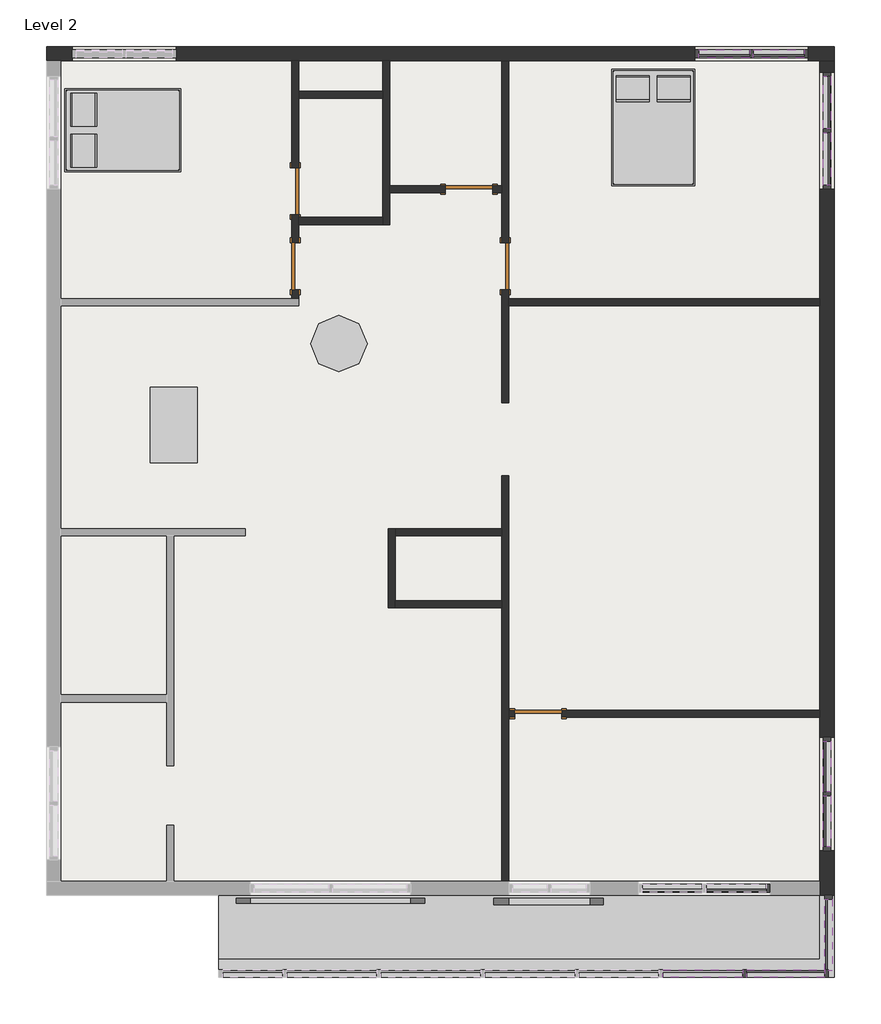
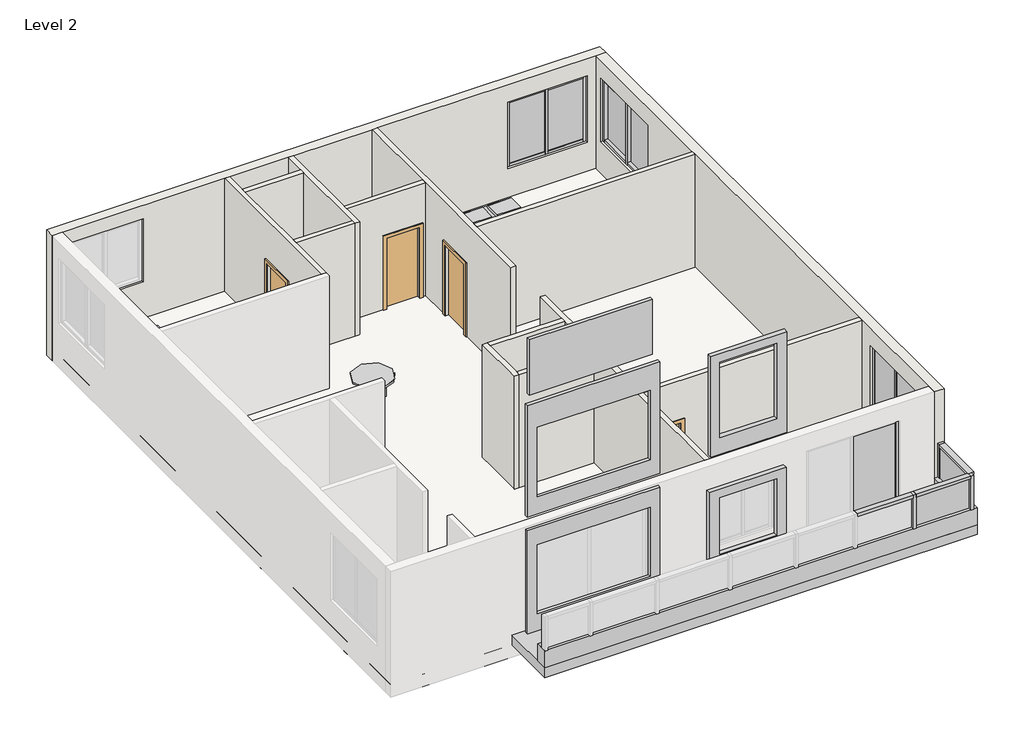
# One storey, part 2 of 2: 30 members, 14 walls, 9 plates, 5 doors, 4 furniture elements, 3 proxies, 1 roof.
"""IFC4 building model written with IfcOpenShell, lengths in millimetres."""

from ifc_helpers import new_model, si_unit, frame, origin, place, context, project, spatial, polyline, outline, extrude, faceted_brep, transform, mapped, element, save
from components import generic_models_10_generic_models_10_e6df43e6, generic_models_11_generic_models_11_8cdfda78, generic_models_4_generic_models_4_9f1effd6, door_f2b275c1, door_d8f5dbb5, furniture_b58f7881, furniture_acc2807d, furniture_52f35bf4, member_c17f1be2, member_7ceeb836, member_9efbbc5c, member_8b2b7717, member_31190633, member_ed313243, member_872f6578, member_8cf20c82, member_801a2072, member_dae9f1c3, member_bf3bc0fd, member_a6f19fa4, member_8ac64e86, member_d7462ea5, member_4edd9ee4, member_1e0ac351, system_panel_glazed_171f6735, system_panel_glazed_e9dc8a15, system_panel_glazed_abee1f72, system_panel_glazed_a27b9eb0, system_panel_glazed_117fd4c3, system_panel_glazed_6fb9d5dc

model = new_model("IFC4")

# Units and contexts
model_context = context("Model", 3, world=origin())
ifc_project = project(units=[si_unit("LENGTHUNIT", "METRE", prefix="MILLI")], contexts=[model_context])

# Site, building, storey
site = spatial("IfcSite", under=ifc_project)
building = spatial("IfcBuilding", under=site)
storey = spatial("IfcBuildingStorey", under=building, Name="Level 2", Elevation=3048.0)

# Proxies
placement = place(None, origin())
generic_models_10_generic_models_10_shape = generic_models_10_generic_models_10_e6df43e6(model_context)
element("IfcBuildingElementProxy", 1, Name="Generic Models 10 : Generic Models 10", ObjectType="Generic Models 10 : Generic Models 10", at=placement, inside=storey, context=model_context, shape_type="MappedRepresentation", body=[
    mapped(generic_models_10_generic_models_10_shape, transform((0.0, 0.0, 0.0), x_axis=(1.0, 0.0, 0.0), y_axis=(0.0, 1.0, 0.0), z_axis=(0.0, 0.0, 1.0))),
])
generic_models_11_generic_models_11_shape = generic_models_11_generic_models_11_8cdfda78(model_context)
element("IfcBuildingElementProxy", 2, Name="Generic Models 11 : Generic Models 11", ObjectType="Generic Models 11 : Generic Models 11", at=placement, inside=storey, context=model_context, shape_type="MappedRepresentation", body=[
    mapped(generic_models_11_generic_models_11_shape, transform((0.0, 0.0, 0.0), x_axis=(1.0, 0.0, 0.0), y_axis=(0.0, 1.0, 0.0), z_axis=(0.0, 0.0, 1.0))),
])
generic_models_4_generic_models_4_shape = generic_models_4_generic_models_4_9f1effd6(model_context)
element("IfcBuildingElementProxy", 3, Name="Generic Models 4 : Generic Models 4", ObjectType="Generic Models 4 : Generic Models 4", at=placement, inside=storey, context=model_context, shape_type="MappedRepresentation", body=[
    mapped(generic_models_4_generic_models_4_shape, transform((0.0, 0.0, 0.0), x_axis=(1.0, 0.0, 0.0), y_axis=(0.0, 1.0, 0.0), z_axis=(0.0, 0.0, 1.0))),
])

# Doors
door_shape = door_f2b275c1(model_context)
element("IfcDoor", 4, ObjectType="Single-Flush : 30\" x 80\"", at=placement, inside=storey, context=model_context, shape_type="MappedRepresentation", body=[
    mapped(door_shape, transform((-14978.0695233, -3968.4252569, 3048.0), x_axis=(0.0, -1.0, 0.0), y_axis=(1.0, 0.0, 0.0), z_axis=(0.0, 0.0, 1.0))),
])
element("IfcDoor", 5, ObjectType="Single-Flush : 30\" x 80\"", at=placement, inside=storey, context=model_context, shape_type="MappedRepresentation", body=[
    mapped(door_shape, transform((-11053.7695233, -11201.0752569, 3048.0), x_axis=(-1.0, 0.0, 0.0), y_axis=(0.0, -1.0, 0.0), z_axis=(0.0, 0.0, 1.0))),
])
door_2_shape = door_d8f5dbb5(model_context)
element("IfcDoor", 6, ObjectType="Single-Flush : 30\" x 80\"", at=placement, inside=storey, context=model_context, shape_type="MappedRepresentation", body=[
    mapped(door_2_shape, transform((-14978.0695233, -2755.5752569, 3048.0), x_axis=(0.0, -1.0, 0.0), y_axis=(1.0, 0.0, 0.0), z_axis=(0.0, 0.0, 1.0))),
])
element("IfcDoor", 7, ObjectType="Single-Flush : 30\" x 80\"", at=placement, inside=storey, context=model_context, shape_type="MappedRepresentation", body=[
    mapped(door_2_shape, transform((-12171.3695233, -2723.8252569, 3048.0), x_axis=(1.0, 0.0, 0.0), y_axis=(0.0, 1.0, 0.0), z_axis=(0.0, 0.0, 1.0))),
])
element("IfcDoor", 8, ObjectType="Single-Flush : 30\" x 80\"", at=placement, inside=storey, context=model_context, shape_type="MappedRepresentation", body=[
    mapped(door_2_shape, transform((-11587.1695233, -3968.4252569, 3048.0), x_axis=(0.0, -1.0, 0.0), y_axis=(1.0, 0.0, 0.0), z_axis=(0.0, 0.0, 1.0))),
])

# Furniture
furniture_shape = furniture_b58f7881(model_context)
element("IfcFurniture", 9, ObjectType="Bed-Box : Double 53\" x 74\"", at=placement, inside=storey, context=model_context, shape_type="MappedRepresentation", body=[
    mapped(furniture_shape, transform((-18000.1490315, -2110.4777159, 3048.0), x_axis=(0.0, 1.0, 0.0), y_axis=(-1.0, 0.0, 0.0), z_axis=(0.0, 0.0, 1.0))),
])
element("IfcFurniture", 10, ObjectType="Bed-Box : Double 53\" x 74\"", at=placement, inside=storey, context=model_context, shape_type="MappedRepresentation", body=[
    mapped(furniture_shape, transform((-9532.3719823, -1492.4457487, 3048.0), x_axis=(1.0, 0.0, 0.0), y_axis=(0.0, 1.0, 0.0), z_axis=(0.0, 0.0, 1.0))),
])
furniture_2_shape = furniture_acc2807d(model_context)
element("IfcFurniture", 11, ObjectType="Table-Coffee Rectangular : 48\" x 30\"", at=placement, inside=storey, context=model_context, shape_type="MappedRepresentation", body=[
    mapped(furniture_2_shape, transform((-16570.6086915, -7147.1588872, 3048.0), x_axis=(0.0, 1.0, 0.0), y_axis=(-1.0, 0.0, 0.0), z_axis=(0.0, 0.0, 1.0))),
])
furniture_3_shape = furniture_52f35bf4(model_context)
element("IfcFurniture", 12, ObjectType="Table-Dining Round w Chairs : 36\" Diameter", at=placement, inside=storey, context=model_context, shape_type="MappedRepresentation", body=[
    mapped(furniture_3_shape, transform((-14376.9014905, -5034.4965684, 3048.0), x_axis=(1.0, 0.0, 0.0), y_axis=(0.0, 1.0, 0.0), z_axis=(0.0, 0.0, 1.0))),
])

# Members
member_shape = member_c17f1be2(model_context)
element("IfcMember", 13, ObjectType="Rectangular Mullion : 2.5\" x 5\" rectangular", at=placement, inside=storey, context=model_context, shape_type="MappedRepresentation", body=[
    mapped(member_shape, transform((-6386.5195233, -12528.2252569, 5666.1206618), x_axis=(0.0, 0.0, 1.0), y_axis=(1.0, 0.0, 0.0), z_axis=(0.0, 1.0, 0.0))),
])
element("IfcMember", 14, ObjectType="Rectangular Mullion : 2.5\" x 5\" rectangular", at=placement, inside=storey, context=model_context, shape_type="MappedRepresentation", body=[
    mapped(member_shape, transform((-6386.5195233, -11645.5752569, 5666.1206618), x_axis=(0.0, 0.0, 1.0), y_axis=(1.0, 0.0, 0.0), z_axis=(0.0, 1.0, 0.0))),
])
element("IfcMember", 15, ObjectType="Rectangular Mullion : 2.5\" x 5\" rectangular", at=placement, inside=storey, context=model_context, shape_type="MappedRepresentation", body=[
    mapped(member_shape, transform((-7573.9695233, -533.0752569, 5665.5630384), x_axis=(0.0, 0.0, 1.0), y_axis=(0.0, 1.0, 0.0), z_axis=(-1.0, 0.0, 0.0))),
])
element("IfcMember", 16, ObjectType="Rectangular Mullion : 2.5\" x 5\" rectangular", at=placement, inside=storey, context=model_context, shape_type="MappedRepresentation", body=[
    mapped(member_shape, transform((-8456.6195233, -533.0752569, 5665.5630384), x_axis=(0.0, 0.0, 1.0), y_axis=(0.0, 1.0, 0.0), z_axis=(-1.0, 0.0, 0.0))),
])
element("IfcMember", 17, ObjectType="Rectangular Mullion : 2.5\" x 5\" rectangular", at=placement, inside=storey, context=model_context, shape_type="MappedRepresentation", body=[
    mapped(member_shape, transform((-6386.5195233, -12464.7252569, 4092.4481408), x_axis=(0.0, 0.0, -1.0), y_axis=(1.0, 0.0, 0.0), z_axis=(0.0, -1.0, 0.0))),
])
element("IfcMember", 18, ObjectType="Rectangular Mullion : 2.5\" x 5\" rectangular", at=placement, inside=storey, context=model_context, shape_type="MappedRepresentation", body=[
    mapped(member_shape, transform((-6386.5195233, -13347.3752569, 4092.4481408), x_axis=(0.0, 0.0, -1.0), y_axis=(1.0, 0.0, 0.0), z_axis=(0.0, -1.0, 0.0))),
])
element("IfcMember", 19, ObjectType="Rectangular Mullion : 2.5\" x 5\" rectangular", at=placement, inside=storey, context=model_context, shape_type="MappedRepresentation", body=[
    mapped(member_shape, transform((-7637.4695233, -533.0752569, 4055.4970292), x_axis=(0.0, 0.0, -1.0), y_axis=(0.0, 1.0, 0.0), z_axis=(1.0, 0.0, 0.0))),
])
element("IfcMember", 20, ObjectType="Rectangular Mullion : 2.5\" x 5\" rectangular", at=placement, inside=storey, context=model_context, shape_type="MappedRepresentation", body=[
    mapped(member_shape, transform((-6754.8195233, -533.0752569, 4055.4970292), x_axis=(0.0, 0.0, -1.0), y_axis=(0.0, 1.0, 0.0), z_axis=(1.0, 0.0, 0.0))),
])
member_2_shape = member_7ceeb836(model_context)
element("IfcMember", 21, ObjectType="Rectangular Mullion : 2.5\" x 5\" rectangular", at=placement, inside=storey, context=model_context, shape_type="MappedRepresentation", body=[
    mapped(member_2_shape, transform((-6386.5195233, -12496.4752569, 4092.4481408), x_axis=(0.0, 1.0, 0.0), y_axis=(1.0, 0.0, 0.0), z_axis=(0.0, 0.0, -1.0))),
])
member_3_shape = member_9efbbc5c(model_context)
element("IfcMember", 22, ObjectType="Rectangular Mullion : 2.5\" x 5\" rectangular", at=placement, inside=storey, context=model_context, shape_type="MappedRepresentation", body=[
    mapped(member_3_shape, transform((-6386.5195233, -11582.0752569, 4092.4481408), x_axis=(0.0, 1.0, 0.0), y_axis=(1.0, 0.0, 0.0), z_axis=(0.0, 0.0, -1.0))),
])
element("IfcMember", 23, ObjectType="Rectangular Mullion : 2.5\" x 5\" rectangular", at=placement, inside=storey, context=model_context, shape_type="MappedRepresentation", body=[
    mapped(member_3_shape, transform((-6386.5195233, -13410.8752569, 5666.1206618), x_axis=(0.0, -1.0, 0.0), y_axis=(1.0, 0.0, 0.0), z_axis=(0.0, 0.0, 1.0))),
])
member_4_shape = member_8b2b7717(model_context)
element("IfcMember", 24, ObjectType="Rectangular Mullion : 2.5\" x 5\" rectangular", at=placement, inside=storey, context=model_context, shape_type="MappedRepresentation", body=[
    mapped(member_4_shape, transform((-6386.5195233, -1749.1002569, 5662.3065021), x_axis=(0.0, 0.0, 1.0), y_axis=(-1.0, 0.0, 0.0), z_axis=(0.0, -1.0, 0.0))),
])
element("IfcMember", 25, ObjectType="Rectangular Mullion : 2.5\" x 5\" rectangular", at=placement, inside=storey, context=model_context, shape_type="MappedRepresentation", body=[
    mapped(member_4_shape, transform((-6386.5195233, -2660.3252569, 5662.3065021), x_axis=(0.0, 0.0, 1.0), y_axis=(-1.0, 0.0, 0.0), z_axis=(0.0, -1.0, 0.0))),
])
member_5_shape = member_31190633(model_context)
element("IfcMember", 26, ObjectType="Rectangular Mullion : 2.5\" x 5\" rectangular", at=placement, inside=storey, context=model_context, shape_type="MappedRepresentation", body=[
    mapped(member_5_shape, transform((-6386.5195233, -1780.8502569, 4118.2676492), x_axis=(0.0, -1.0, 0.0), y_axis=(-1.0, 0.0, 0.0), z_axis=(0.0, 0.0, -1.0))),
])
element("IfcMember", 27, ObjectType="Rectangular Mullion : 2.5\" x 5\" rectangular", at=placement, inside=storey, context=model_context, shape_type="MappedRepresentation", body=[
    mapped(member_4_shape, transform((-6386.5195233, -1812.6002569, 4118.2676492), x_axis=(0.0, 0.0, -1.0), y_axis=(-1.0, 0.0, 0.0), z_axis=(0.0, 1.0, 0.0))),
])
element("IfcMember", 28, ObjectType="Rectangular Mullion : 2.5\" x 5\" rectangular", at=placement, inside=storey, context=model_context, shape_type="MappedRepresentation", body=[
    mapped(member_4_shape, transform((-6386.5195233, -901.3752569, 4118.2676492), x_axis=(0.0, 0.0, -1.0), y_axis=(-1.0, 0.0, 0.0), z_axis=(0.0, 1.0, 0.0))),
])
member_6_shape = member_ed313243(model_context)
element("IfcMember", 29, ObjectType="Rectangular Mullion : 2.5\" x 5\" rectangular", at=placement, inside=storey, context=model_context, shape_type="MappedRepresentation", body=[
    mapped(member_6_shape, transform((-6386.5195233, -837.8752569, 5662.3065021), x_axis=(0.0, 1.0, 0.0), y_axis=(-1.0, 0.0, 0.0), z_axis=(0.0, 0.0, 1.0))),
])
element("IfcMember", 30, ObjectType="Rectangular Mullion : 2.5\" x 5\" rectangular", at=placement, inside=storey, context=model_context, shape_type="MappedRepresentation", body=[
    mapped(member_6_shape, transform((-6386.5195233, -2723.8252569, 4118.2676492), x_axis=(0.0, -1.0, 0.0), y_axis=(-1.0, 0.0, 0.0), z_axis=(0.0, 0.0, -1.0))),
])
member_7_shape = member_872f6578(model_context)
element("IfcMember", 31, ObjectType="Rectangular Mullion : 2.5\" x 5\" rectangular", at=placement, inside=storey, context=model_context, shape_type="MappedRepresentation", body=[
    mapped(member_7_shape, transform((-7605.7195233, -533.0752569, 4055.4970292), x_axis=(-1.0, 0.0, 0.0), y_axis=(0.0, 1.0, 0.0), z_axis=(0.0, 0.0, -1.0))),
])
member_8_shape = member_8cf20c82(model_context)
element("IfcMember", 32, ObjectType="Rectangular Mullion : 2.5\" x 5\" rectangular", at=placement, inside=storey, context=model_context, shape_type="MappedRepresentation", body=[
    mapped(member_8_shape, transform((-8520.1195233, -533.0752569, 4055.4970292), x_axis=(-1.0, 0.0, 0.0), y_axis=(0.0, 1.0, 0.0), z_axis=(0.0, 0.0, -1.0))),
])
element("IfcMember", 33, ObjectType="Rectangular Mullion : 2.5\" x 5\" rectangular", at=placement, inside=storey, context=model_context, shape_type="MappedRepresentation", body=[
    mapped(member_8_shape, transform((-6691.3195233, -533.0752569, 5665.5630384), x_axis=(1.0, 0.0, 0.0), y_axis=(0.0, 1.0, 0.0), z_axis=(0.0, 0.0, 1.0))),
])
member_9_shape = member_801a2072(model_context)
element("IfcMember", 34, ObjectType="Rectangular Mullion : 2.5\" x 5\" rectangular", at=placement, inside=storey, context=model_context, shape_type="MappedRepresentation", body=[
    mapped(member_9_shape, transform((-8399.4695233, -14020.4752569, 3693.4399111), x_axis=(0.0, 0.0, -1.0), y_axis=(0.0, 1.0, 0.0), z_axis=(1.0, 0.0, 0.0))),
])
element("IfcMember", 35, ObjectType="Rectangular Mullion : 2.5\" x 5\" rectangular", at=placement, inside=storey, context=model_context, shape_type="MappedRepresentation", body=[
    mapped(member_9_shape, transform((-7364.4195233, -14020.4752569, 3693.4399111), x_axis=(0.0, 0.0, -1.0), y_axis=(0.0, 1.0, 0.0), z_axis=(1.0, 0.0, 0.0))),
])
member_10_shape = member_dae9f1c3(model_context)
element("IfcMember", 36, ObjectType="Rectangular Mullion : 2.5\" x 5\" rectangular", at=placement, inside=storey, context=model_context, shape_type="MappedRepresentation", body=[
    mapped(member_10_shape, transform((-7300.9195233, -14020.4752569, 5682.139627), x_axis=(1.0, 0.0, 0.0), y_axis=(0.0, 1.0, 0.0), z_axis=(0.0, 0.0, 1.0))),
])
member_11_shape = member_bf3bc0fd(model_context)
element("IfcMember", 37, ObjectType="Rectangular Mullion : 2.5\" x 5\" rectangular", at=placement, inside=storey, context=model_context, shape_type="MappedRepresentation", body=[
    mapped(member_11_shape, transform((-7748.4379121, -15398.1130528, 4822.8286641), x_axis=(0.0, 0.0, 1.0), y_axis=(0.0, -1.0, 0.0), z_axis=(1.0, 0.0, 0.0))),
])
member_12_shape = member_a6f19fa4(model_context)
element("IfcMember", 38, ObjectType="Rectangular Mullion : 2.5\" x 5\" rectangular", at=placement, inside=storey, context=model_context, shape_type="MappedRepresentation", body=[
    mapped(member_12_shape, transform((-6425.5212454, -15398.1130528, 4822.8286641), x_axis=(0.0, 0.0, 1.0), y_axis=(0.0, -1.0, 0.0), z_axis=(1.0, 0.0, 0.0))),
])
member_13_shape = member_8ac64e86(model_context)
element("IfcMember", 39, ObjectType="Rectangular Mullion : 2.5\" x 5\" rectangular", at=placement, inside=storey, context=model_context, shape_type="MappedRepresentation", body=[
    mapped(member_13_shape, transform((-6362.0212454, -15398.1130528, 4001.8016497), x_axis=(1.0, 0.0, 0.0), y_axis=(0.0, -1.0, 0.0), z_axis=(0.0, 0.0, -1.0))),
])
member_14_shape = member_d7462ea5(model_context)
element("IfcMember", 40, ObjectType="Rectangular Mullion : 2.5\" x 5\" rectangular", at=placement, inside=storey, context=model_context, shape_type="MappedRepresentation", body=[
    mapped(member_14_shape, transform((-7716.6879121, -15398.1130528, 4001.8016497), x_axis=(1.0, 0.0, 0.0), y_axis=(0.0, -1.0, 0.0), z_axis=(0.0, 0.0, -1.0))),
])
member_15_shape = member_4edd9ee4(model_context)
element("IfcMember", 41, ObjectType="Rectangular Mullion : 2.5\" x 5\" rectangular", at=placement, inside=storey, context=model_context, shape_type="MappedRepresentation", body=[
    mapped(member_15_shape, transform((-6362.0212454, -14134.7752569, 4001.8016497), x_axis=(0.0, 1.0, 0.0), y_axis=(1.0, 0.0, 0.0), z_axis=(0.0, 0.0, -1.0))),
])
member_16_shape = member_1e0ac351(model_context)
element("IfcMember", 42, ObjectType="Rectangular Mullion : 2.5\" x 5\" rectangular", at=placement, inside=storey, context=model_context, shape_type="MappedRepresentation", body=[
    mapped(member_16_shape, transform((-6362.0212454, -14198.2752569, 4825.345459), x_axis=(0.0, 0.0, 1.0), y_axis=(1.0, 0.0, 0.0), z_axis=(0.0, 1.0, 0.0))),
])

# Plates
system_panel_glazed_shape = system_panel_glazed_171f6735(model_context)
element("IfcPlate", 43, ObjectType="System Panel : Glazed", at=placement, inside=storey, context=model_context, shape_type="MappedRepresentation", body=[
    mapped(system_panel_glazed_shape, transform((-6386.5195233, -12937.8002569, 4155.9481408), x_axis=(0.0, 1.0, 0.0), y_axis=(-1.0, 0.0, 0.0), z_axis=(0.0, 0.0, 1.0))),
])
element("IfcPlate", 44, ObjectType="System Panel : Glazed", at=placement, inside=storey, context=model_context, shape_type="MappedRepresentation", body=[
    mapped(system_panel_glazed_shape, transform((-6386.5195233, -12055.1502569, 4155.9481408), x_axis=(0.0, 1.0, 0.0), y_axis=(-1.0, 0.0, 0.0), z_axis=(0.0, 0.0, 1.0))),
])
system_panel_glazed_2_shape = system_panel_glazed_e9dc8a15(model_context)
element("IfcPlate", 45, ObjectType="System Panel : Glazed", at=placement, inside=storey, context=model_context, shape_type="MappedRepresentation", body=[
    mapped(system_panel_glazed_2_shape, transform((-6386.5195233, -1325.2377569, 4181.7676492), x_axis=(0.0, -1.0, 0.0), y_axis=(1.0, 0.0, 0.0), z_axis=(0.0, 0.0, 1.0))),
])
element("IfcPlate", 46, ObjectType="System Panel : Glazed", at=placement, inside=storey, context=model_context, shape_type="MappedRepresentation", body=[
    mapped(system_panel_glazed_2_shape, transform((-6386.5195233, -2236.4627569, 4181.7676492), x_axis=(0.0, -1.0, 0.0), y_axis=(1.0, 0.0, 0.0), z_axis=(0.0, 0.0, 1.0))),
])
system_panel_glazed_3_shape = system_panel_glazed_abee1f72(model_context)
element("IfcPlate", 47, ObjectType="System Panel : Glazed", at=placement, inside=storey, context=model_context, shape_type="MappedRepresentation", body=[
    mapped(system_panel_glazed_3_shape, transform((-7164.3945233, -533.0752569, 4118.9970292), x_axis=(-1.0, 0.0, 0.0), y_axis=(0.0, -1.0, 0.0), z_axis=(0.0, 0.0, 1.0))),
])
element("IfcPlate", 48, ObjectType="System Panel : Glazed", at=placement, inside=storey, context=model_context, shape_type="MappedRepresentation", body=[
    mapped(system_panel_glazed_3_shape, transform((-8047.0445233, -533.0752569, 4118.9970292), x_axis=(-1.0, 0.0, 0.0), y_axis=(0.0, -1.0, 0.0), z_axis=(0.0, 0.0, 1.0))),
])
system_panel_glazed_4_shape = system_panel_glazed_a27b9eb0(model_context)
element("IfcPlate", 49, ObjectType="System Panel : Glazed", at=placement, inside=storey, context=model_context, shape_type="MappedRepresentation", body=[
    mapped(system_panel_glazed_4_shape, transform((-7850.1945233, -14020.4752569, 3756.9399111), x_axis=(-1.0, 0.0, 0.0), y_axis=(0.0, -1.0, 0.0), z_axis=(0.0, 0.0, 1.0))),
])
system_panel_glazed_5_shape = system_panel_glazed_117fd4c3(model_context)
element("IfcPlate", 50, ObjectType="System Panel : Glazed", at=placement, inside=storey, context=model_context, shape_type="MappedRepresentation", body=[
    mapped(system_panel_glazed_5_shape, transform((-7055.2295788, -15398.1130528, 4001.8016497), x_axis=(1.0, 0.0, 0.0), y_axis=(0.0, 1.0, 0.0), z_axis=(0.0, 0.0, 1.0))),
])
system_panel_glazed_6_shape = system_panel_glazed_6fb9d5dc(model_context)
element("IfcPlate", 51, ObjectType="System Panel : Glazed", at=placement, inside=storey, context=model_context, shape_type="MappedRepresentation", body=[
    mapped(system_panel_glazed_6_shape, transform((-6362.0212454, -14775.9691549, 4001.8016497), x_axis=(0.0, 1.0, 0.0), y_axis=(-1.0, 0.0, 0.0), z_axis=(0.0, 0.0, 1.0))),
])

# Roof
element("IfcRoof", 52, ObjectType="Generic - 12\"", at=placement, inside=storey, context=model_context, shape_type="SweptSolid", body=[
    extrude(outline(polyline([(-18997.6195233, -418.7752569), (-6272.2195233, -418.7752569), (-6272.2195233, -14134.7752569), (-18997.6195233, -14134.7752569), (-18997.6195233, -418.7752569)])), frame((0.0, 0.0, 3048.0), z_axis=(0.0, 0.0, 1.0), x_axis=(1.0, 0.0, 0.0)), (0.0, 0.0, 1.0), 304.8),
])

# Walls
element("IfcWall", 53, ObjectType="4.5\"", at=placement, inside=storey, context=model_context, shape_type="Brep", body=[
    faceted_brep([(-11530.0195233, -13906.1752569, 3048.0), (-11530.0195233, -11258.2252569, 3048.0), (-11530.0195233, -11143.9252569, 3048.0), (-11530.0195233, -7352.9752569, 3048.0), (-11530.0195233, -7352.9752569, 6096.0), (-11530.0195233, -11143.9252569, 6096.0), (-11530.0195233, -11258.2252569, 6096.0), (-11530.0195233, -13906.1752569, 6096.0), (-11644.3195233, -13906.1752569, 3048.0), (-11644.3195233, -13906.1752569, 6096.0), (-11644.3195233, -9486.5752569, 6096.0), (-11644.3195233, -9372.2752569, 6096.0), (-11644.3195233, -8324.5252569, 6096.0), (-11644.3195233, -8210.2252569, 6096.0), (-11644.3195233, -7352.9752569, 6096.0), (-11644.3195233, -7352.9752569, 3048.0), (-11644.3195233, -8210.2252569, 3048.0), (-11644.3195233, -8324.5252569, 3048.0), (-11644.3195233, -9372.2752569, 3048.0), (-11644.3195233, -9486.5752569, 3048.0)], [[[0, 1, 2, 3, 4, 5, 6, 7]], [[8, 9, 10, 11, 12, 13, 14, 15, 16, 17, 18, 19]], [[3, 2, 1, 0, 8, 19, 18, 17, 16, 15]], [[4, 3, 15, 14]], [[7, 6, 5, 4, 14, 13, 12, 11, 10, 9]], [[0, 7, 9, 8]]]),
])
element("IfcWall", 54, ObjectType="4.5\"", at=placement, inside=storey, context=model_context, shape_type="SweptSolid", body=[
    extrude(outline(polyline([(3048.0, -11530.0195233), (3048.0, -11434.7695233), (5080.0, -11434.7695233), (5080.0, -10672.7695233), (3048.0, -10672.7695233), (3048.0, -6500.8195233), (6096.0, -6500.8195233), (6096.0, -11530.0195233), (3048.0, -11530.0195233)])), frame((0.0, -11258.2252569, 0.0), z_axis=(0.0, 1.0, 0.0), x_axis=(0.0, 0.0, 1.0)), (0.0, 0.0, 1.0), 114.3),
])
element("IfcWall", 55, ObjectType="4.5\"", at=placement, inside=storey, context=model_context, shape_type="Brep", body=[
    faceted_brep([(-14920.9195233, -3587.4252569, 3048.0), (-14920.9195233, -3295.3252569, 3048.0), (-14920.9195233, -3181.0252569, 3048.0), (-14920.9195233, -3136.5752569, 3048.0), (-14920.9195233, -3136.5752569, 5080.0), (-14920.9195233, -2374.5752569, 5080.0), (-14920.9195233, -2374.5752569, 3048.0), (-14920.9195233, -1256.9752569, 3048.0), (-14920.9195233, -1142.6752569, 3048.0), (-14920.9195233, -647.3752569, 3048.0), (-14920.9195233, -647.3752569, 6096.0), (-14920.9195233, -1142.6752569, 6096.0), (-14920.9195233, -1256.9752569, 6096.0), (-14920.9195233, -3181.0252569, 6096.0), (-14920.9195233, -3295.3252569, 6096.0), (-14920.9195233, -4495.4752569, 6096.0), (-14920.9195233, -4495.4752569, 3048.0), (-14920.9195233, -4349.4252569, 3048.0), (-14920.9195233, -4349.4252569, 5080.0), (-14920.9195233, -3587.4252569, 5080.0), (-15035.2195233, -3136.5752569, 5080.0), (-15035.2195233, -3136.5752569, 3048.0), (-15035.2195233, -3587.4252569, 3048.0), (-15035.2195233, -3587.4252569, 5080.0), (-15035.2195233, -4349.4252569, 5080.0), (-15035.2195233, -4349.4252569, 3048.0), (-15035.2195233, -4495.4752569, 3048.0), (-15035.2195233, -4495.4752569, 6096.0), (-15035.2195233, -647.3752569, 6096.0), (-15035.2195233, -647.3752569, 3048.0), (-15035.2195233, -2374.5752569, 3048.0), (-15035.2195233, -2374.5752569, 5080.0)], [[[0, 1, 2, 3, 4, 5, 6, 7, 8, 9, 10, 11, 12, 13, 14, 15, 16, 17, 18, 19]], [[20, 21, 22, 23, 24, 25, 26, 27, 28, 29, 30, 31]], [[26, 25, 17, 16]], [[30, 29, 9, 8, 7, 6]], [[22, 21, 3, 2, 1, 0]], [[15, 14, 13, 12, 11, 10, 28, 27]], [[16, 15, 27, 26]], [[10, 9, 29, 28]], [[18, 17, 25, 24]], [[19, 18, 24, 23]], [[0, 19, 23, 22]], [[4, 3, 21, 20]], [[5, 4, 20, 31]], [[6, 5, 31, 30]]]),
])
element("IfcWall", 56, ObjectType="4.5\"", at=placement, inside=storey, context=model_context, shape_type="SweptSolid", body=[
    extrude(outline(polyline([(-13568.3695233, -1256.9752569), (-14920.9195233, -1256.9752569), (-14920.9195233, -1142.6752569), (-13568.3695233, -1142.6752569), (-13568.3695233, -1256.9752569)])), frame((0.0, 0.0, 3048.0), z_axis=(0.0, 0.0, 1.0), x_axis=(1.0, 0.0, 0.0)), (0.0, 0.0, 1.0), 3048.0),
])
element("IfcWall", 57, ObjectType="4.5\"", at=placement, inside=storey, context=model_context, shape_type="Brep", body=[
    faceted_brep([(-13454.0695233, -3295.3252569, 3048.0), (-13454.0695233, -2780.9752569, 3048.0), (-13454.0695233, -2666.6752569, 3048.0), (-13454.0695233, -647.3752569, 3048.0), (-13454.0695233, -647.3752569, 6096.0), (-13454.0695233, -2666.6752569, 6096.0), (-13454.0695233, -2780.9752569, 6096.0), (-13454.0695233, -3295.3252569, 6096.0), (-13568.3695233, -3295.3252569, 3048.0), (-13568.3695233, -3295.3252569, 6096.0), (-13568.3695233, -3181.0252569, 6096.0), (-13568.3695233, -1256.9752569, 6096.0), (-13568.3695233, -1142.6752569, 6096.0), (-13568.3695233, -647.3752569, 6096.0), (-13568.3695233, -647.3752569, 3048.0), (-13568.3695233, -1142.6752569, 3048.0), (-13568.3695233, -1256.9752569, 3048.0), (-13568.3695233, -3181.0252569, 3048.0)], [[[0, 1, 2, 3, 4, 5, 6, 7]], [[8, 9, 10, 11, 12, 13, 14, 15, 16, 17]], [[3, 2, 1, 0, 8, 17, 16, 15, 14]], [[7, 6, 5, 4, 13, 12, 11, 10, 9]], [[4, 3, 14, 13]], [[0, 7, 9, 8]]]),
])
element("IfcWall", 58, ObjectType="4.5\"", at=placement, inside=storey, context=model_context, shape_type="SweptSolid", body=[
    extrude(outline(polyline([(-14920.9195233, -3181.0252569), (-13568.3695233, -3181.0252569), (-13568.3695233, -3295.3252569), (-14920.9195233, -3295.3252569), (-14920.9195233, -3181.0252569)])), frame((0.0, 0.0, 3048.0), z_axis=(0.0, 0.0, 1.0), x_axis=(1.0, 0.0, 0.0)), (0.0, 0.0, 1.0), 3048.0),
])
element("IfcWall", 59, ObjectType="4.5\"", at=placement, inside=storey, context=model_context, shape_type="SweptSolid", body=[
    extrude(outline(polyline([(5080.0, -11790.3695233), (3048.0, -11790.3695233), (3048.0, -11644.3195233), (6096.0, -11644.3195233), (6096.0, -13454.0695233), (3048.0, -13454.0695233), (3048.0, -12552.3695233), (5080.0, -12552.3695233), (5080.0, -11790.3695233)])), frame((0.0, -2780.9752569, 0.0), z_axis=(0.0, 1.0, 0.0), x_axis=(0.0, 0.0, 1.0)), (0.0, 0.0, 1.0), 114.3),
])
element("IfcWall", 60, ObjectType="4.5\"", at=placement, inside=storey, context=model_context, shape_type="Brep", body=[
    faceted_brep([(-11530.0195233, -6178.2252569, 3048.0), (-11530.0195233, -4609.7752569, 3048.0), (-11530.0195233, -4495.4752569, 3048.0), (-11530.0195233, -4349.4252569, 3048.0), (-11530.0195233, -4349.4252569, 5080.0), (-11530.0195233, -3587.4252569, 5080.0), (-11530.0195233, -3587.4252569, 3048.0), (-11530.0195233, -647.3752569, 3048.0), (-11530.0195233, -647.3752569, 6096.0), (-11530.0195233, -4495.4752569, 6096.0), (-11530.0195233, -4609.7752569, 6096.0), (-11530.0195233, -6178.2252569, 6096.0), (-11644.3195233, -4349.4252569, 5080.0), (-11644.3195233, -4349.4252569, 3048.0), (-11644.3195233, -6178.2252569, 3048.0), (-11644.3195233, -6178.2252569, 6096.0), (-11644.3195233, -2780.9752569, 6096.0), (-11644.3195233, -2666.6752569, 6096.0), (-11644.3195233, -647.3752569, 6096.0), (-11644.3195233, -647.3752569, 3048.0), (-11644.3195233, -2666.6752569, 3048.0), (-11644.3195233, -2780.9752569, 3048.0), (-11644.3195233, -3587.4252569, 3048.0), (-11644.3195233, -3587.4252569, 5080.0)], [[[0, 1, 2, 3, 4, 5, 6, 7, 8, 9, 10, 11]], [[12, 13, 14, 15, 16, 17, 18, 19, 20, 21, 22, 23]], [[14, 13, 3, 2, 1, 0]], [[22, 21, 20, 19, 7, 6]], [[11, 10, 9, 8, 18, 17, 16, 15]], [[0, 11, 15, 14]], [[8, 7, 19, 18]], [[4, 3, 13, 12]], [[5, 4, 12, 23]], [[6, 5, 23, 22]]]),
])
element("IfcWall", 61, ObjectType="4.5\"", at=placement, inside=storey, context=model_context, shape_type="SweptSolid", body=[
    extrude(outline(polyline([(-6500.8195233, -4609.7752569), (-11530.0195233, -4609.7752569), (-11530.0195233, -4495.4752569), (-6500.8195233, -4495.4752569), (-6500.8195233, -4609.7752569)])), frame((0.0, 0.0, 3048.0), z_axis=(0.0, 0.0, 1.0), x_axis=(1.0, 0.0, 0.0)), (0.0, 0.0, 1.0), 3048.0),
])
element("IfcWall", 62, ObjectType="4.5\"", at=placement, inside=storey, context=model_context, shape_type="Brep", body=[
    faceted_brep([(-13473.1195233, -8210.2252569, 3048.0), (-13473.1195233, -9486.5752569, 3048.0), (-13473.1195233, -9486.5752569, 6096.0), (-13473.1195233, -8210.2252569, 6096.0), (-13358.8195233, -8210.2252569, 3048.0), (-13358.8195233, -8210.2252569, 6096.0), (-13358.8195233, -8324.5252569, 6096.0), (-13358.8195233, -9372.2752569, 6096.0), (-13358.8195233, -9486.5752569, 6096.0), (-13358.8195233, -9486.5752569, 3048.0), (-13358.8195233, -9372.2752569, 3048.0), (-13358.8195233, -8324.5252569, 3048.0)], [[[0, 1, 2, 3]], [[4, 5, 6, 7, 8, 9, 10, 11]], [[1, 0, 4, 11, 10, 9]], [[3, 2, 8, 7, 6, 5]], [[2, 1, 9, 8]], [[0, 3, 5, 4]]]),
])
element("IfcWall", 63, ObjectType="4.5\"", at=placement, inside=storey, context=model_context, shape_type="SweptSolid", body=[
    extrude(outline(polyline([(-11644.3195233, -9486.5752569), (-13358.8195233, -9486.5752569), (-13358.8195233, -9372.2752569), (-11644.3195233, -9372.2752569), (-11644.3195233, -9486.5752569)])), frame((0.0, 0.0, 3048.0), z_axis=(0.0, 0.0, 1.0), x_axis=(1.0, 0.0, 0.0)), (0.0, 0.0, 1.0), 3048.0),
])
element("IfcWall", 64, ObjectType="4.5\"", at=placement, inside=storey, context=model_context, shape_type="SweptSolid", body=[
    extrude(outline(polyline([(-11644.3195233, -8324.5252569), (-13358.8195233, -8324.5252569), (-13358.8195233, -8210.2252569), (-11644.3195233, -8210.2252569), (-11644.3195233, -8324.5252569)])), frame((0.0, 0.0, 3048.0), z_axis=(0.0, 0.0, 1.0), x_axis=(1.0, 0.0, 0.0)), (0.0, 0.0, 1.0), 3048.0),
])
element("IfcWall", 65, ObjectType="9\"", at=placement, inside=storey, context=model_context, shape_type="Brep", body=[
    faceted_brep([(-18997.6195233, -647.3752569, 3048.0), (-18769.0195233, -647.3752569, 3048.0), (-15035.2195233, -647.3752569, 3048.0), (-14920.9195233, -647.3752569, 3048.0), (-13568.3695233, -647.3752569, 3048.0), (-13454.0695233, -647.3752569, 3048.0), (-11644.3195233, -647.3752569, 3048.0), (-11530.0195233, -647.3752569, 3048.0), (-6500.8195233, -647.3752569, 3048.0), (-6272.2195233, -647.3752569, 3048.0), (-6272.2195233, -647.3752569, 6096.0), (-6500.8195233, -647.3752569, 6096.0), (-11530.0195233, -647.3752569, 6096.0), (-11644.3195233, -647.3752569, 6096.0), (-13454.0695233, -647.3752569, 6096.0), (-13568.3695233, -647.3752569, 6096.0), (-14920.9195233, -647.3752569, 6096.0), (-15035.2195233, -647.3752569, 6096.0), (-18769.0195233, -647.3752569, 6096.0), (-18997.6195233, -647.3752569, 6096.0), (-6691.3195233, -647.3752569, 5665.5630384), (-6691.3195233, -647.3752569, 4055.4970292), (-8520.1195233, -647.3752569, 4055.4970292), (-8520.1195233, -647.3752569, 5665.5630384), (-18578.5195233, -647.3752569, 4232.1728983), (-18578.5195233, -647.3752569, 5767.2358325), (-16902.1195233, -647.3752569, 5767.2358325), (-16902.1195233, -647.3752569, 4232.1728983), (-6272.2195233, -418.7752569, 3048.0), (-18997.6195233, -418.7752569, 3048.0), (-18997.6195233, -418.7752569, 6096.0), (-6272.2195233, -418.7752569, 6096.0), (-6691.3195233, -418.7752569, 4055.4970292), (-6691.3195233, -418.7752569, 5665.5630384), (-8520.1195233, -418.7752569, 5665.5630384), (-8520.1195233, -418.7752569, 4055.4970292), (-18578.5195233, -418.7752569, 5767.2358325), (-18578.5195233, -418.7752569, 4232.1728983), (-16902.1195233, -418.7752569, 4232.1728983), (-16902.1195233, -418.7752569, 5767.2358325)], [[[0, 1, 2, 3, 4, 5, 6, 7, 8, 9, 10, 11, 12, 13, 14, 15, 16, 17, 18, 19], [20, 21, 22, 23], [24, 25, 26, 27]], [[28, 29, 30, 31], [32, 33, 34, 35], [36, 37, 38, 39]], [[9, 8, 7, 6, 5, 4, 3, 2, 1, 0, 29, 28]], [[19, 18, 17, 16, 15, 14, 13, 12, 11, 10, 31, 30]], [[10, 9, 28, 31]], [[0, 19, 30, 29]], [[32, 21, 20, 33]], [[33, 20, 23, 34]], [[34, 23, 22, 35]], [[21, 32, 35, 22]], [[36, 25, 24, 37]], [[25, 36, 39, 26]], [[26, 39, 38, 27]], [[37, 24, 27, 38]]]),
])
element("IfcWall", 66, ObjectType="9\"", at=placement, inside=storey, context=model_context, shape_type="Brep", body=[
    faceted_brep([(-6272.2195233, -14134.7752569, 3048.0), (-6272.2195233, -647.3752569, 3048.0), (-6272.2195233, -647.3752569, 6096.0), (-6272.2195233, -14134.7752569, 6096.0), (-6272.2195233, -13410.8752569, 4092.4481408), (-6272.2195233, -13410.8752569, 5666.1206618), (-6272.2195233, -11582.0752569, 5666.1206618), (-6272.2195233, -11582.0752569, 4092.4481408), (-6272.2195233, -837.8752569, 5662.3065021), (-6272.2195233, -837.8752569, 4118.2676492), (-6272.2195233, -2723.8252569, 4118.2676492), (-6272.2195233, -2723.8252569, 5662.3065021), (-6500.8195233, -647.3752569, 3048.0), (-6500.8195233, -4495.4752569, 3048.0), (-6500.8195233, -4609.7752569, 3048.0), (-6500.8195233, -11143.9252569, 3048.0), (-6500.8195233, -11258.2252569, 3048.0), (-6500.8195233, -13906.1752569, 3048.0), (-6500.8195233, -14134.7752569, 3048.0), (-6500.8195233, -14134.7752569, 6096.0), (-6500.8195233, -13906.1752569, 6096.0), (-6500.8195233, -11258.2252569, 6096.0), (-6500.8195233, -11143.9252569, 6096.0), (-6500.8195233, -4609.7752569, 6096.0), (-6500.8195233, -4495.4752569, 6096.0), (-6500.8195233, -647.3752569, 6096.0), (-6500.8195233, -13410.8752569, 5666.1206618), (-6500.8195233, -13410.8752569, 4092.4481408), (-6500.8195233, -11582.0752569, 4092.4481408), (-6500.8195233, -11582.0752569, 5666.1206618), (-6500.8195233, -837.8752569, 4118.2676492), (-6500.8195233, -837.8752569, 5662.3065021), (-6500.8195233, -2723.8252569, 5662.3065021), (-6500.8195233, -2723.8252569, 4118.2676492)], [[[0, 1, 2, 3], [4, 5, 6, 7], [8, 9, 10, 11]], [[12, 13, 14, 15, 16, 17, 18, 19, 20, 21, 22, 23, 24, 25], [26, 27, 28, 29], [30, 31, 32, 33]], [[1, 0, 18, 17, 16, 15, 14, 13, 12]], [[3, 2, 25, 24, 23, 22, 21, 20, 19]], [[2, 1, 12, 25]], [[0, 3, 19, 18]], [[4, 27, 26, 5]], [[5, 26, 29, 6]], [[6, 29, 28, 7]], [[27, 4, 7, 28]], [[30, 9, 8, 31]], [[31, 8, 11, 32]], [[10, 33, 32, 11]], [[9, 30, 33, 10]]]),
])

save(model, "model.ifc")

# Revit data of these elements
# Type "Single-Flush : 30\" x 80\""
#   Type Mark = "5"
#   Construction Type Id = "MDOOR"
#   Assembly Code = "C1020"
#   Analytic Construction = "Metal"
#   Thickness = 0' - 2"
#   Heat Transfer Coefficient (U) = 0.651978 BTU/(h·ft²·°F)
#   Height = 6' - 8"
#   Trim Projection Ext = 0' - 1"
#   Trim Projection Int = 0' - 1"
#   Trim Width = 0' - 3"
#   Width = 2' - 6"
#   Define Thermal Properties by = 1
#   Define Thermal Properties by = 1
#   Door Material = Door - Panel
#   Frame Material = Door - Frame
#   Visual Light Transmittance = 0
#   Solar Heat Gain Coefficient = 0
#   Function = (empty or 0)
#   Wall Closure = (empty or 0)
# Type "Bed-Box : Double 53\" x 74\""
#   Assembly Code = "E2020200"
#   Length = 6' - 2"
#   Width = 4' - 5"
#   Frame Material = Birch
#   Mattress Material = Linen, White
#   Default Elevation = 0
# Type "Table-Coffee Rectangular : 48\" x 30\""
#   Assembly Code = "E2020200"
#   Height = 1' - 1"
#   Length = 4' - 0"
#   Width = 2' - 6"
#   Base Material = Metal - Chrome
#   Table Top Material = Glass - Clear, Grey
#   Default Elevation = 0
# Type "Table-Dining Round w Chairs : 36\" Diameter"
#   Assembly Code = "E2020200"
#   Radius = 1' - 6"
#   Diameter = 3' - 0"
#   Height = 2' - 6"
#   Chairs = 4
#   Base Material = Pine
#   Top Material = Laminate, Linen, Matte
#   Default Elevation = 0
# Type "Rectangular Mullion : 2.5\" x 5\" rectangular"
#   built-in parameter 1007304 = 0.416667 (stored number, unit not read)
#   built-in parameter 1007301 = 0.104167 (stored number, unit not read)
#   built-in parameter 1007300 = 0.104167 (stored number, unit not read)
# Type "System Panel : Glazed"
#   Construction Type Id = "GSP4R"
#   Analytic Construction = "1/8 in Pilkington single glazing"
#   Visual Light Transmittance = 0.9
#   Solar Heat Gain Coefficient = 0.86
#   Heat Transfer Coefficient (U) = 1.18115 BTU/(h·ft²·°F)
#   Define Thermal Properties by = 1
# Type "Generic - 12\""
#   Assembly Code = "B1020"
#   Layers, outside or top first: 1' - 0" no material (function 1)
# Type "4.5\""
#   Assembly Code = "B2010"
#   Layers, outside or top first: 0' - 4 1/2" no material (function 1)
# Type "9\""
#   Assembly Code = "B2010"
#   Layers, outside or top first: 0' - 9" no material (function 1)
# Element 1 (IfcBuildingElementProxy, "Generic Models 10 : Generic Models 10")
#   Phase Created = New Construction
# Element 2 (IfcBuildingElementProxy, "Generic Models 11 : Generic Models 11")
#   Phase Created = New Construction
# Element 3 (IfcBuildingElementProxy, "Generic Models 4 : Generic Models 4")
#   Phase Created = New Construction
# Elements 4, 5, 6, 7, 8 (IfcDoor, "Single-Flush : 30\" x 80\"")
#   Phase Created = New Construction
#   Materials on its faces: "Door - Frame", "Door - Panel"
# Elements 9, 10 (IfcFurniture, "Bed-Box : Double 53\" x 74\"")
#   Phase Created = New Construction
#   Materials on its faces: "Birch", "Linen, White"
# Element 11 (IfcFurniture, "Table-Coffee Rectangular : 48\" x 30\"")
#   Phase Created = New Construction
#   Materials on its faces: "Metal - Chrome", "Glass - Clear, Grey"
# Element 12 (IfcFurniture, "Table-Dining Round w Chairs : 36\" Diameter")
#   Phase Created = New Construction
#   Materials on its faces: "Pine", "Laminate, Linen, Matte"
# Elements 13, 14, 15, 16, 17, 18, 19, 20, 21, 22, 23, 24, 25, 26, 27, 28, 29, 30, 31, 32, 33, 34, 35, 36, 37, 38, 39, 40, 41, 42 (IfcMember, "Rectangular Mullion : 2.5\" x 5\" rectangular")
#   Phase Created = New Construction
#   Materials on its faces: "Aluminum"
# Elements 43, 44, 45, 46, 47, 48, 49, 50, 51 (IfcPlate, "System Panel : Glazed")
#   Phase Created = New Construction
#   Materials on its faces: "Glass"
# Element 52 (IfcRoof, "Generic - 12\"")
#   built-in parameter 1001705 = 11 (stored number, unit not read)
#   built-in parameter 1001710 = 33615
#   Phase Created = New Construction
#   Materials on its faces: "Default Roof"
# Elements 53, 54, 55, 56, 57, 58, 59, 60, 61, 62, 63, 64 (IfcWall, "4.5\"")
#   Top Offset = 0' - 0"
#   Base Offset = 0' - 0"
#   Unconnected Height = 10' - 0"
#   wall height = 10' - 0"
#   Phase Created = New Construction
#   Base Constraint = Level 2
#   Materials on its faces: "Default Wall"
# Elements 65, 66 (IfcWall, "9\"")
#   Top Offset = 0' - 0"
#   Base Offset = 0' - 0"
#   Unconnected Height = 10' - 0"
#   wall height = 10' - 0"
#   Phase Created = New Construction
#   Base Constraint = Level 2
#   Materials on its faces: "Default Wall"
# Materials
#   "Door - Panel": class "Wood", colour RGB 210 159 95, transparency 0, Cost = 0
#   "Door - Frame": colour RGB 118 70 51, transparency 0, Cost = 0
#   "Birch": class "Wood", colour RGB 224 178 126, transparency 0, Description = "Betula Alleghaniensis", Cost = 0
#   "Linen, White": class "Textile", colour RGB 247 247 239, transparency 0, Description = "Linen, white", Cost = 0
#   "Metal - Chrome": colour RGB 57 57 57, transparency 0
#   "Glass - Clear, Grey": colour RGB 252 255 255, transparency 0.64
#   "Pine": class "Wood", colour RGB 223 192 134, transparency 0, Description = "Pinus Echinata", Cost = 0
#   "Laminate, Linen, Matte": class "Plastic", colour RGB 249 239 230, transparency 0, Description = "Plastic Laminate - Linen, Matte", Cost = 0
#   "Aluminum": class "Metal", colour RGB 247 247 247, transparency 0, Description = "Aluminum 6061", Cost = 0
#   "Glass": class "Glass", colour RGB 0 128 192, transparency 0.75, Description = "Soda Lime Glass", Cost = 0
#   "Default Roof": colour RGB 88 101 114, transparency 0, Cost = 0
#   "Default Wall": colour RGB 128 128 128, transparency 0, Cost = 0
